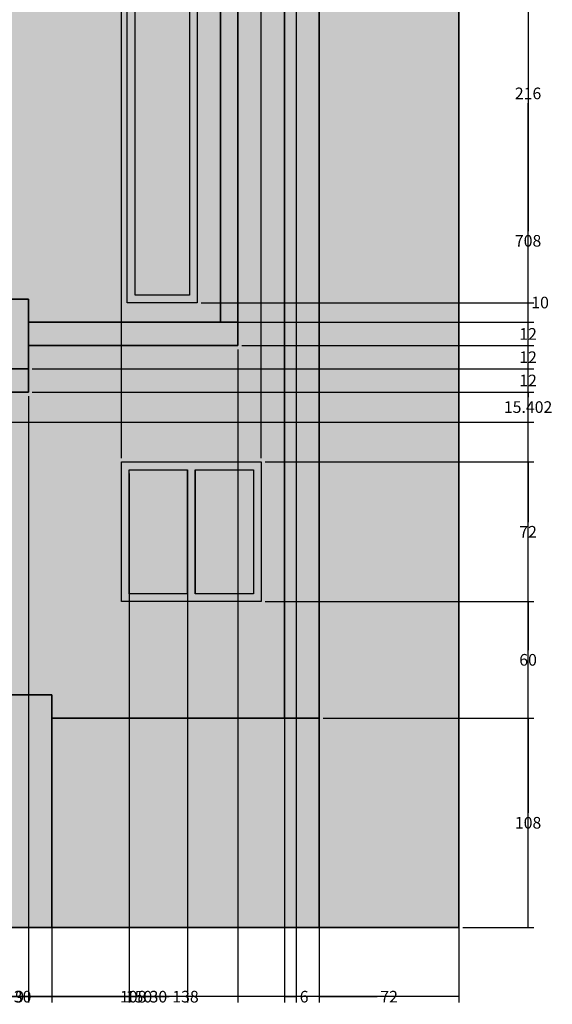
# Model space of a CAD drawing. Units: inches. Extents: x 860 to 1491, y 583 to 1370.
# Tile 6 of 8: x 1216 to 1491, y 583 to 1091. Entities that reach past the tile are written whole.
import ezdxf

# ---------------------------------------------------------------- set-up
doc = ezdxf.new("R2010")
doc.units = ezdxf.units.IN
doc.header["$MEASUREMENT"] = 0
doc.layers.get('0').update_dxf_attribs({"color": 250})
for name, color, linetype, lineweight in [('A-ANNO-DIMS', 2, 'Continuous', 18), ('A-ELEV', 7, 'Continuous', 35), ('A-ELEV-PATT', 9, 'Continuous', 13), ('A-GLAZ', 4, 'Continuous', 25), ('A-GLAZ-PATT', 150, 'Continuous', 13), ('A-SITE-PATT', 8, 'Continuous', 13), ('A-SITE-WALL', 7, 'Continuous', 35)]:
    doc.layers.add(name, color=color, linetype=linetype, lineweight=lineweight)
doc.styles.get("Standard").update_dxf_attribs({"font": 'arial.ttf'})
doc.dimstyles.get("Standard").update_dxf_attribs({"dimtxt": 6, "dimasz": 0.18, "dimexe": 3, "dimexo": 2, "dimgap": 2, "dimtad": 0, "dimtih": 1, "dimtoh": 1, "dimdec": 0, "dimzin": 0, "dimdsep": 46, "dimlunit": 3, "dimtxsty": 'Standard', "dimblk2": 'CLOSEDBLANK', "dimsah": 1, "dimcen": 2, "dimadec": 0, "dimazin": 0, "dimtfac": 1, "dimtdec": 0, "dimtofl": 0, "dimtmove": 0, "dimatfit": 3, "dimfxl": 1, "dimtolj": 1, "dimtzin": 0, "dimarcsym": 0})

# ---------------------------------------------------------------- blocks, each defined once
blk = doc.blocks.new('_ClosedBlank')
at = {"color": 0, "linetype": 'ByBlock', "lineweight": -2}
for p, q in [((-1, 0.17), (0, 0)), ((-1, 0.17), (-1, -0.17)), ((0, 0), (-1, -0.17))]:
    blk.add_line(p, q, dxfattribs=at)
blk = doc.blocks.new('*D2')
at = {"layer": 'A-ANNO-DIMS', "color": 0, "lineweight": -2, "transparency": 16777216}
for p, q in [((1442.44, 1328.76), (1442.44, 584.11)), ((908.34, 740.76), (908.34, 584.11)), ((908.52, 587.11), (1163.85, 587.11)), ((1442.26, 587.11), (1186.93, 587.11))]:
    blk.add_line(p, q, dxfattribs=at)
at = {"layer": 'A-ANNO-DIMS', "color": 0, "transparency": 16777216}
blk.add_solid([(908.52, 587.14), (908.52, 587.08), (908.34, 587.11)], dxfattribs=at)
at = {"layer": 'Defpoints', "color": 0, "transparency": 16777216}
for p in [(1442.44, 1330.76), (908.34, 742.76), (1442.44, 587.11)]:
    blk.add_point(p, dxfattribs=at)
at = {"layer": 'A-ANNO-DIMS', "color": 0, "lineweight": -2, "transparency": 16777216, "xscale": 0.18, "yscale": 0.18, "zscale": 0.18}
blk.add_blockref('_ClosedBlank', (1442.44, 587.11), dxfattribs=at)
at = {"layer": 'A-ANNO-DIMS', "color": 0, "transparency": 16777216, "insert": (1175.39, 587.11), "char_height": 6, "attachment_point": 5}
blk.add_mtext('\\A1;534.1', dxfattribs=at)
blk = doc.blocks.new('*D3')
at = {"layer": 'A-ANNO-DIMS', "color": 0, "lineweight": -2, "transparency": 16777216}
for p, q in [((1444.44, 1330.76), (1481.09, 1330.76)), ((1478.09, 1330.58), (1478.09, 981.82)), ((1478.09, 622.94), (1478.09, 971.69)), ((1444.44, 622.76), (1481.09, 622.76))]:
    blk.add_line(p, q, dxfattribs=at)
at = {"layer": 'A-ANNO-DIMS', "color": 0, "transparency": 16777216}
blk.add_solid([(1478.06, 622.94), (1478.12, 622.94), (1478.09, 622.76)], dxfattribs=at)
at = {"layer": 'Defpoints', "color": 0, "transparency": 16777216}
for p in [(1442.44, 1330.76), (1478.09, 1330.76), (1442.44, 622.76)]:
    blk.add_point(p, dxfattribs=at)
at = {"layer": 'A-ANNO-DIMS', "color": 0, "lineweight": -2, "transparency": 16777216, "xscale": 0.18, "yscale": 0.18, "zscale": 0.18, "rotation": 90}
blk.add_blockref('_ClosedBlank', (1478.09, 1330.76), dxfattribs=at)
at = {"layer": 'A-ANNO-DIMS', "color": 0, "transparency": 16777216, "insert": (1478.09, 976.76), "char_height": 6, "attachment_point": 5}
blk.add_mtext('\\A1;708', dxfattribs=at)
blk = doc.blocks.new('*D17')
at = {"layer": 'A-ANNO-DIMS', "color": 0, "lineweight": -2, "transparency": 16777216}
for p, q in [((1202.44, 740.76), (1202.44, 584.11)), ((1232.44, 740.76), (1232.44, 584.11)), ((1202.62, 587.11), (1211.16, 587.11)), ((1232.26, 587.11), (1223.73, 587.11))]:
    blk.add_line(p, q, dxfattribs=at)
at = {"layer": 'A-ANNO-DIMS', "color": 0, "transparency": 16777216}
blk.add_solid([(1202.62, 587.14), (1202.62, 587.08), (1202.44, 587.11)], dxfattribs=at)
at = {"layer": 'Defpoints', "color": 0, "transparency": 16777216}
for p in [(1202.44, 742.76), (1232.44, 742.76), (1232.44, 587.11)]:
    blk.add_point(p, dxfattribs=at)
at = {"layer": 'A-ANNO-DIMS', "color": 0, "lineweight": -2, "transparency": 16777216, "xscale": 0.18, "yscale": 0.18, "zscale": 0.18}
blk.add_blockref('_ClosedBlank', (1232.44, 587.11), dxfattribs=at)
at = {"layer": 'A-ANNO-DIMS', "color": 0, "transparency": 16777216, "insert": (1217.44, 587.11), "char_height": 6, "attachment_point": 5}
blk.add_mtext('\\A1;30', dxfattribs=at)
blk = doc.blocks.new('*D18')
at = {"layer": 'A-ANNO-DIMS', "color": 0, "lineweight": -2, "transparency": 16777216}
for p, q in [((1232.44, 740.76), (1232.44, 584.11)), ((1370.44, 728.76), (1370.44, 584.11)), ((1232.62, 587.11), (1293.09, 587.11)), ((1370.26, 587.11), (1309.79, 587.11))]:
    blk.add_line(p, q, dxfattribs=at)
at = {"layer": 'A-ANNO-DIMS', "color": 0, "transparency": 16777216}
blk.add_solid([(1232.62, 587.14), (1232.62, 587.08), (1232.44, 587.11)], dxfattribs=at)
at = {"layer": 'Defpoints', "color": 0, "transparency": 16777216}
for p in [(1232.44, 742.76), (1370.44, 730.76), (1370.44, 587.11)]:
    blk.add_point(p, dxfattribs=at)
at = {"layer": 'A-ANNO-DIMS', "color": 0, "lineweight": -2, "transparency": 16777216, "xscale": 0.18, "yscale": 0.18, "zscale": 0.18}
blk.add_blockref('_ClosedBlank', (1370.44, 587.11), dxfattribs=at)
at = {"layer": 'A-ANNO-DIMS', "color": 0, "transparency": 16777216, "insert": (1301.44, 587.11), "char_height": 6, "attachment_point": 5}
blk.add_mtext('\\A1;138', dxfattribs=at)
blk = doc.blocks.new('*D19')
at = {"layer": 'A-ANNO-DIMS', "color": 0, "lineweight": -2, "transparency": 16777216}
for p, q in [((1370.44, 728.76), (1370.44, 584.11)), ((1442.44, 620.76), (1442.44, 584.11)), ((1370.62, 587.11), (1400.2, 587.11)), ((1442.26, 587.11), (1412.68, 587.11))]:
    blk.add_line(p, q, dxfattribs=at)
at = {"layer": 'A-ANNO-DIMS', "color": 0, "transparency": 16777216}
blk.add_solid([(1370.62, 587.14), (1370.62, 587.08), (1370.44, 587.11)], dxfattribs=at)
at = {"layer": 'Defpoints', "color": 0, "transparency": 16777216}
for p in [(1370.44, 730.76), (1442.44, 622.76), (1442.44, 587.11)]:
    blk.add_point(p, dxfattribs=at)
at = {"layer": 'A-ANNO-DIMS', "color": 0, "lineweight": -2, "transparency": 16777216, "xscale": 0.18, "yscale": 0.18, "zscale": 0.18}
blk.add_blockref('_ClosedBlank', (1442.44, 587.11), dxfattribs=at)
at = {"layer": 'A-ANNO-DIMS', "color": 0, "transparency": 16777216, "insert": (1406.44, 587.11), "char_height": 6, "attachment_point": 5}
blk.add_mtext('\\A1;72', dxfattribs=at)
blk = doc.blocks.new('*D26')
at = {"layer": 'A-ANNO-DIMS', "color": 0, "lineweight": -2, "transparency": 16777216}
for p, q in [((1202.44, 744.76), (1202.44, 1369.41)), ((1202.62, 1366.41), (1229.13, 1366.41)), ((1268.26, 1366.41), (1241.75, 1366.41)), ((1268.44, 864.76), (1268.44, 1369.41))]:
    blk.add_line(p, q, dxfattribs=at)
at = {"layer": 'A-ANNO-DIMS', "color": 0, "transparency": 16777216}
blk.add_solid([(1202.62, 1366.44), (1202.62, 1366.38), (1202.44, 1366.41)], dxfattribs=at)
at = {"layer": 'Defpoints', "color": 0, "transparency": 16777216}
for p in [(1268.44, 1366.41), (1268.44, 862.76), (1202.44, 742.76)]:
    blk.add_point(p, dxfattribs=at)
at = {"layer": 'A-ANNO-DIMS', "color": 0, "lineweight": -2, "transparency": 16777216, "xscale": 0.18, "yscale": 0.18, "zscale": 0.18}
blk.add_blockref('_ClosedBlank', (1268.44, 1366.41), dxfattribs=at)
at = {"layer": 'A-ANNO-DIMS', "color": 0, "transparency": 16777216, "insert": (1235.44, 1366.41), "char_height": 6, "attachment_point": 5}
blk.add_mtext('\\A1;66', dxfattribs=at)
blk = doc.blocks.new('*D27')
at = {"layer": 'A-ANNO-DIMS', "color": 0, "lineweight": -2, "transparency": 16777216}
for p, q in [((1268.44, 864.76), (1268.44, 1369.41)), ((1268.62, 1366.41), (1298.2, 1366.41)), ((1340.26, 1366.41), (1310.68, 1366.41)), ((1340.44, 864.76), (1340.44, 1369.41))]:
    blk.add_line(p, q, dxfattribs=at)
at = {"layer": 'A-ANNO-DIMS', "color": 0, "transparency": 16777216}
blk.add_solid([(1268.62, 1366.44), (1268.62, 1366.38), (1268.44, 1366.41)], dxfattribs=at)
at = {"layer": 'Defpoints', "color": 0, "transparency": 16777216}
for p in [(1340.44, 1366.41), (1268.44, 862.76), (1340.44, 862.76)]:
    blk.add_point(p, dxfattribs=at)
at = {"layer": 'A-ANNO-DIMS', "color": 0, "lineweight": -2, "transparency": 16777216, "xscale": 0.18, "yscale": 0.18, "zscale": 0.18}
blk.add_blockref('_ClosedBlank', (1340.44, 1366.41), dxfattribs=at)
at = {"layer": 'A-ANNO-DIMS', "color": 0, "transparency": 16777216, "insert": (1304.44, 1366.41), "char_height": 6, "attachment_point": 5}
blk.add_mtext('\\A1;72', dxfattribs=at)
blk = doc.blocks.new('*D28')
at = {"layer": 'A-ANNO-DIMS', "color": 0, "lineweight": -2, "transparency": 16777216}
for p, q in [((1340.260309, 1366.405507), (1340.080309, 1366.405507)), ((1340.440309, 864.755507), (1340.440309, 1369.405507)), ((1352.440309, 732.755507), (1352.440309, 1369.405507)), ((1352.620309, 1366.405507), (1352.800309, 1366.405507))]:
    blk.add_line(p, q, dxfattribs=at)
at = {"layer": 'A-ANNO-DIMS', "color": 0, "transparency": 16777216}
blk.add_solid([(1340.260309, 1366.435507), (1340.260309, 1366.375507), (1340.440309, 1366.405507)], dxfattribs=at)
at = {"layer": 'Defpoints', "color": 0, "transparency": 16777216}
for p in [(1352.440309, 1366.405507), (1340.440309, 862.755507), (1352.440309, 730.755507)]:
    blk.add_point(p, dxfattribs=at)
at = {"layer": 'A-ANNO-DIMS', "color": 0, "lineweight": -2, "transparency": 16777216, "xscale": 0.18, "yscale": 0.18, "zscale": 0.18, "rotation": 180}
blk.add_blockref('_ClosedBlank', (1352.440309, 1366.405507), dxfattribs=at)
at = {"layer": 'A-ANNO-DIMS', "color": 0, "transparency": 16777216, "insert": (1346.440309, 1366.405507), "char_height": 6, "attachment_point": 5}
blk.add_mtext('\\A1;12', dxfattribs=at)
blk = doc.blocks.new('*D29')
at = {"layer": 'A-ANNO-DIMS', "color": 0, "lineweight": -2, "transparency": 16777216}
for p, q in [((1352.44, 732.76), (1352.44, 1369.41)), ((1352.62, 1366.41), (1355.42, 1366.41)), ((1370.26, 1366.41), (1367.46, 1366.41)), ((1370.44, 732.76), (1370.44, 1369.41))]:
    blk.add_line(p, q, dxfattribs=at)
at = {"layer": 'A-ANNO-DIMS', "color": 0, "transparency": 16777216}
blk.add_solid([(1352.62, 1366.44), (1352.62, 1366.38), (1352.44, 1366.41)], dxfattribs=at)
at = {"layer": 'Defpoints', "color": 0, "transparency": 16777216}
for p in [(1370.44, 1366.41), (1352.44, 730.76), (1370.44, 730.76)]:
    blk.add_point(p, dxfattribs=at)
at = {"layer": 'A-ANNO-DIMS', "color": 0, "lineweight": -2, "transparency": 16777216, "xscale": 0.18, "yscale": 0.18, "zscale": 0.18}
blk.add_blockref('_ClosedBlank', (1370.44, 1366.41), dxfattribs=at)
at = {"layer": 'A-ANNO-DIMS', "color": 0, "transparency": 16777216, "insert": (1361.44, 1366.41), "char_height": 6, "attachment_point": 5}
blk.add_mtext('\\A1;18', dxfattribs=at)
blk = doc.blocks.new('*D30')
at = {"layer": 'A-ANNO-DIMS', "color": 0, "lineweight": -2, "transparency": 16777216}
for p, q in [((1272.44, 856.76), (1272.44, 584.11)), ((1302.44, 856.76), (1302.44, 584.11)), ((1272.62, 587.11), (1281.16, 587.11)), ((1302.26, 587.11), (1293.73, 587.11))]:
    blk.add_line(p, q, dxfattribs=at)
at = {"layer": 'A-ANNO-DIMS', "color": 0, "transparency": 16777216}
blk.add_solid([(1272.62, 587.14), (1272.62, 587.08), (1272.44, 587.11)], dxfattribs=at)
at = {"layer": 'Defpoints', "color": 0, "transparency": 16777216}
for p in [(1272.44, 858.76), (1302.44, 858.76), (1302.44, 587.11)]:
    blk.add_point(p, dxfattribs=at)
at = {"layer": 'A-ANNO-DIMS', "color": 0, "lineweight": -2, "transparency": 16777216, "xscale": 0.18, "yscale": 0.18, "zscale": 0.18}
blk.add_blockref('_ClosedBlank', (1302.44, 587.11), dxfattribs=at)
at = {"layer": 'A-ANNO-DIMS', "color": 0, "transparency": 16777216, "insert": (1287.44, 587.11), "char_height": 6, "attachment_point": 5}
blk.add_mtext('\\A1;30', dxfattribs=at)
blk = doc.blocks.new('*D36')
at = {"layer": 'A-ANNO-DIMS', "color": 0, "lineweight": -2, "transparency": 16777216}
for p, q in [((1372.44, 730.76), (1481.09, 730.76)), ((1478.09, 730.58), (1478.09, 681.82)), ((1478.09, 622.94), (1478.09, 671.69)), ((1444.44, 622.76), (1481.09, 622.76))]:
    blk.add_line(p, q, dxfattribs=at)
at = {"layer": 'A-ANNO-DIMS', "color": 0, "transparency": 16777216}
blk.add_solid([(1478.06, 622.94), (1478.12, 622.94), (1478.09, 622.76)], dxfattribs=at)
at = {"layer": 'Defpoints', "color": 0, "transparency": 16777216}
for p in [(1370.44, 730.76), (1478.09, 730.76), (1442.44, 622.76)]:
    blk.add_point(p, dxfattribs=at)
at = {"layer": 'A-ANNO-DIMS', "color": 0, "lineweight": -2, "transparency": 16777216, "xscale": 0.18, "yscale": 0.18, "zscale": 0.18, "rotation": 90}
blk.add_blockref('_ClosedBlank', (1478.09, 730.76), dxfattribs=at)
at = {"layer": 'A-ANNO-DIMS', "color": 0, "transparency": 16777216, "insert": (1478.09, 676.76), "char_height": 6, "attachment_point": 5}
blk.add_mtext('\\A1;108', dxfattribs=at)
blk = doc.blocks.new('*D37')
at = {"layer": 'A-ANNO-DIMS', "color": 0, "lineweight": -2, "transparency": 16777216}
for p, q in [((1342.44, 790.76), (1481.09, 790.76)), ((1478.09, 790.58), (1478.09, 765.82)), ((1478.09, 730.94), (1478.09, 755.69)), ((1372.44, 730.76), (1481.09, 730.76))]:
    blk.add_line(p, q, dxfattribs=at)
at = {"layer": 'A-ANNO-DIMS', "color": 0, "transparency": 16777216}
blk.add_solid([(1478.06, 730.94), (1478.12, 730.94), (1478.09, 730.76)], dxfattribs=at)
at = {"layer": 'Defpoints', "color": 0, "transparency": 16777216}
for p in [(1340.44, 790.76), (1478.09, 790.76), (1370.44, 730.76)]:
    blk.add_point(p, dxfattribs=at)
at = {"layer": 'A-ANNO-DIMS', "color": 0, "lineweight": -2, "transparency": 16777216, "xscale": 0.18, "yscale": 0.18, "zscale": 0.18, "rotation": 90}
blk.add_blockref('_ClosedBlank', (1478.09, 790.76), dxfattribs=at)
at = {"layer": 'A-ANNO-DIMS', "color": 0, "transparency": 16777216, "insert": (1478.09, 760.76), "char_height": 6, "attachment_point": 5}
blk.add_mtext('\\A1;60', dxfattribs=at)
blk = doc.blocks.new('*D38')
at = {"layer": 'A-ANNO-DIMS', "color": 0, "lineweight": -2, "transparency": 16777216}
for p, q in [((1342.44, 862.76), (1481.09, 862.76)), ((1478.09, 862.58), (1478.09, 831.77)), ((1478.09, 790.94), (1478.09, 821.74)), ((1342.44, 790.76), (1481.09, 790.76))]:
    blk.add_line(p, q, dxfattribs=at)
at = {"layer": 'A-ANNO-DIMS', "color": 0, "transparency": 16777216}
blk.add_solid([(1478.06, 790.94), (1478.12, 790.94), (1478.09, 790.76)], dxfattribs=at)
at = {"layer": 'Defpoints', "color": 0, "transparency": 16777216}
for p in [(1340.44, 862.76), (1478.09, 862.76), (1340.44, 790.76)]:
    blk.add_point(p, dxfattribs=at)
at = {"layer": 'A-ANNO-DIMS', "color": 0, "lineweight": -2, "transparency": 16777216, "xscale": 0.18, "yscale": 0.18, "zscale": 0.18, "rotation": 90}
blk.add_blockref('_ClosedBlank', (1478.09, 862.76), dxfattribs=at)
at = {"layer": 'A-ANNO-DIMS', "color": 0, "transparency": 16777216, "insert": (1478.09, 826.76), "char_height": 6, "attachment_point": 5}
blk.add_mtext('\\A1;72', dxfattribs=at)
blk = doc.blocks.new('*D48')
at = {"layer": 'A-ANNO-DIMS', "color": 0, "lineweight": -2, "transparency": 16777216}
for p, q in [((1222.44, 898.76), (1481.09, 898.76)), ((1478.09, 898.58), (1478.09, 896.12)), ((964.34, 883.35), (1481.09, 883.35)), ((1478.09, 883.53), (1478.09, 885.99))]:
    blk.add_line(p, q, dxfattribs=at)
at = {"layer": 'A-ANNO-DIMS', "color": 0, "transparency": 16777216}
blk.add_solid([(1478.06, 883.53), (1478.12, 883.53), (1478.09, 883.35)], dxfattribs=at)
at = {"layer": 'Defpoints', "color": 0, "transparency": 16777216}
for p in [(1220.44, 898.76), (1478.09, 898.76), (962.34, 883.35)]:
    blk.add_point(p, dxfattribs=at)
at = {"layer": 'A-ANNO-DIMS', "color": 0, "lineweight": -2, "transparency": 16777216, "xscale": 0.18, "yscale": 0.18, "zscale": 0.18, "rotation": 90}
blk.add_blockref('_ClosedBlank', (1478.09, 898.76), dxfattribs=at)
at = {"layer": 'A-ANNO-DIMS', "color": 0, "transparency": 16777216, "insert": (1478.09, 891.05), "char_height": 6, "attachment_point": 5}
blk.add_mtext('\\A1;15.402', dxfattribs=at)
blk = doc.blocks.new('*D49')
at = {"layer": 'A-ANNO-DIMS', "color": 0, "lineweight": -2, "transparency": 16777216}
for p, q in [((1222.440309, 910.755507), (1481.090309, 910.755507)), ((1478.090309, 910.935507), (1478.090309, 911.115507)), ((1222.440309, 898.755507), (1481.090309, 898.755507)), ((1478.090309, 898.575507), (1478.090309, 898.395507))]:
    blk.add_line(p, q, dxfattribs=at)
at = {"layer": 'A-ANNO-DIMS', "color": 0, "transparency": 16777216}
blk.add_solid([(1478.060309, 898.575507), (1478.120309, 898.575507), (1478.090309, 898.755507)], dxfattribs=at)
at = {"layer": 'Defpoints', "color": 0, "transparency": 16777216}
for p in [(1220.440309, 910.755507), (1478.090309, 910.755507), (1220.440309, 898.755507)]:
    blk.add_point(p, dxfattribs=at)
at = {"layer": 'A-ANNO-DIMS', "color": 0, "lineweight": -2, "transparency": 16777216, "xscale": 0.18, "yscale": 0.18, "zscale": 0.18, "rotation": 270}
blk.add_blockref('_ClosedBlank', (1478.090309, 910.755507), dxfattribs=at)
at = {"layer": 'A-ANNO-DIMS', "color": 0, "transparency": 16777216, "insert": (1478.090309, 904.755507), "char_height": 6, "attachment_point": 5}
blk.add_mtext('\\A1;12', dxfattribs=at)
blk = doc.blocks.new('*D50')
at = {"layer": 'A-ANNO-DIMS', "color": 0, "lineweight": -2, "transparency": 16777216}
for p, q in [((1330.440309, 922.755507), (1481.090309, 922.755507)), ((1478.090309, 922.935507), (1478.090309, 923.115507)), ((1222.440309, 910.755507), (1481.090309, 910.755507)), ((1478.090309, 910.575507), (1478.090309, 910.395507))]:
    blk.add_line(p, q, dxfattribs=at)
at = {"layer": 'A-ANNO-DIMS', "color": 0, "transparency": 16777216}
blk.add_solid([(1478.060309, 910.575507), (1478.120309, 910.575507), (1478.090309, 910.755507)], dxfattribs=at)
at = {"layer": 'Defpoints', "color": 0, "transparency": 16777216}
for p in [(1328.440309, 922.755507), (1478.090309, 922.755507), (1220.440309, 910.755507)]:
    blk.add_point(p, dxfattribs=at)
at = {"layer": 'A-ANNO-DIMS', "color": 0, "lineweight": -2, "transparency": 16777216, "xscale": 0.18, "yscale": 0.18, "zscale": 0.18, "rotation": 270}
blk.add_blockref('_ClosedBlank', (1478.090309, 922.755507), dxfattribs=at)
at = {"layer": 'A-ANNO-DIMS', "color": 0, "transparency": 16777216, "insert": (1478.090309, 916.755507), "char_height": 6, "attachment_point": 5}
blk.add_mtext('\\A1;12', dxfattribs=at)
blk = doc.blocks.new('*D51')
at = {"layer": 'A-ANNO-DIMS', "color": 0, "lineweight": -2, "transparency": 16777216}
for p, q in [((1321.440309, 934.755507), (1481.090309, 934.755507)), ((1478.090309, 934.935507), (1478.090309, 935.115507)), ((1330.440309, 922.755507), (1481.090309, 922.755507)), ((1478.090309, 922.575507), (1478.090309, 922.395507))]:
    blk.add_line(p, q, dxfattribs=at)
at = {"layer": 'A-ANNO-DIMS', "color": 0, "transparency": 16777216}
blk.add_solid([(1478.060309, 922.575507), (1478.120309, 922.575507), (1478.090309, 922.755507)], dxfattribs=at)
at = {"layer": 'Defpoints', "color": 0, "transparency": 16777216}
for p in [(1319.440309, 934.755507), (1478.090309, 934.755507), (1328.440309, 922.755507)]:
    blk.add_point(p, dxfattribs=at)
at = {"layer": 'A-ANNO-DIMS', "color": 0, "lineweight": -2, "transparency": 16777216, "xscale": 0.18, "yscale": 0.18, "zscale": 0.18, "rotation": 270}
blk.add_blockref('_ClosedBlank', (1478.090309, 934.755507), dxfattribs=at)
at = {"layer": 'A-ANNO-DIMS', "color": 0, "transparency": 16777216, "insert": (1478.090309, 928.755507), "char_height": 6, "attachment_point": 5}
blk.add_mtext('\\A1;12', dxfattribs=at)
blk = doc.blocks.new('*D52')
at = {"layer": 'A-ANNO-DIMS', "color": 0, "lineweight": -2, "transparency": 16777216}
for p, q in [((1309.44, 944.76), (1481.09, 944.76)), ((1478.09, 944.76), (1478.09, 944.94)), ((1478.09, 944.94), (1478.27, 944.94)), ((1478.09, 934.94), (1478.09, 944.58)), ((1321.44, 934.76), (1481.09, 934.76))]:
    blk.add_line(p, q, dxfattribs=at)
at = {"layer": 'A-ANNO-DIMS', "color": 0, "transparency": 16777216}
blk.add_solid([(1478.06, 934.94), (1478.12, 934.94), (1478.09, 934.76)], dxfattribs=at)
at = {"layer": 'Defpoints', "color": 0, "transparency": 16777216}
for p in [(1307.44, 944.76), (1478.09, 944.76), (1319.44, 934.76)]:
    blk.add_point(p, dxfattribs=at)
at = {"layer": 'A-ANNO-DIMS', "color": 0, "lineweight": -2, "transparency": 16777216, "xscale": 0.18, "yscale": 0.18, "zscale": 0.18, "rotation": 90}
blk.add_blockref('_ClosedBlank', (1478.09, 944.76), dxfattribs=at)
at = {"layer": 'A-ANNO-DIMS', "color": 0, "transparency": 16777216, "insert": (1484.28, 944.94), "char_height": 6, "attachment_point": 5}
blk.add_mtext('\\A1;10', dxfattribs=at)
blk = doc.blocks.new('*D53')
at = {"layer": 'A-ANNO-DIMS', "color": 0, "lineweight": -2, "transparency": 16777216}
for p, q in [((1309.44, 1160.76), (1481.09, 1160.76)), ((1478.09, 1160.58), (1478.09, 1057.82)), ((1478.09, 944.94), (1478.09, 1047.69)), ((1309.44, 944.76), (1481.09, 944.76))]:
    blk.add_line(p, q, dxfattribs=at)
at = {"layer": 'A-ANNO-DIMS', "color": 0, "transparency": 16777216}
blk.add_solid([(1478.06, 944.94), (1478.12, 944.94), (1478.09, 944.76)], dxfattribs=at)
at = {"layer": 'Defpoints', "color": 0, "transparency": 16777216}
for p in [(1307.44, 1160.76), (1478.09, 1160.76), (1307.44, 944.76)]:
    blk.add_point(p, dxfattribs=at)
at = {"layer": 'A-ANNO-DIMS', "color": 0, "lineweight": -2, "transparency": 16777216, "xscale": 0.18, "yscale": 0.18, "zscale": 0.18, "rotation": 90}
blk.add_blockref('_ClosedBlank', (1478.09, 1160.76), dxfattribs=at)
at = {"layer": 'A-ANNO-DIMS', "color": 0, "transparency": 16777216, "insert": (1478.09, 1052.76), "char_height": 6, "attachment_point": 5}
blk.add_mtext('\\A1;216', dxfattribs=at)
blk = doc.blocks.new('*D61')
at = {"layer": 'A-ANNO-DIMS', "color": 0, "lineweight": -2, "transparency": 16777216}
for p, q in [((1319.260309, 1366.405507), (1319.080309, 1366.405507)), ((1319.440309, 1186.755507), (1319.440309, 1369.405507)), ((1328.440309, 924.755507), (1328.440309, 1369.405507)), ((1328.620309, 1366.405507), (1328.800309, 1366.405507))]:
    blk.add_line(p, q, dxfattribs=at)
at = {"layer": 'A-ANNO-DIMS', "color": 0, "transparency": 16777216}
blk.add_solid([(1319.260309, 1366.435507), (1319.260309, 1366.375507), (1319.440309, 1366.405507)], dxfattribs=at)
at = {"layer": 'Defpoints', "color": 0, "transparency": 16777216}
for p in [(1328.440309, 1366.405507), (1319.440309, 1184.755507), (1328.440309, 922.755507)]:
    blk.add_point(p, dxfattribs=at)
at = {"layer": 'A-ANNO-DIMS', "color": 0, "lineweight": -2, "transparency": 16777216, "xscale": 0.18, "yscale": 0.18, "zscale": 0.18, "rotation": 180}
blk.add_blockref('_ClosedBlank', (1328.440309, 1366.405507), dxfattribs=at)
at = {"layer": 'A-ANNO-DIMS', "color": 0, "transparency": 16777216, "insert": (1323.940309, 1366.405507), "char_height": 6, "attachment_point": 5}
blk.add_mtext('\\A1;9', dxfattribs=at)
blk = doc.blocks.new('*D69')
at = {"layer": 'A-ANNO-DIMS', "color": 0, "lineweight": -2, "transparency": 16777216}
for p, q in [((1211.440309, 980.755507), (1211.440309, 584.105507)), ((1220.440309, 896.755507), (1220.440309, 584.105507)), ((1211.260309, 587.105507), (1211.080309, 587.105507)), ((1220.620309, 587.105507), (1220.800309, 587.105507))]:
    blk.add_line(p, q, dxfattribs=at)
at = {"layer": 'A-ANNO-DIMS', "color": 0, "transparency": 16777216}
blk.add_solid([(1211.260309, 587.135507), (1211.260309, 587.075507), (1211.440309, 587.105507)], dxfattribs=at)
at = {"layer": 'Defpoints', "color": 0, "transparency": 16777216}
for p in [(1211.440309, 982.755507), (1220.440309, 898.755507), (1220.440309, 587.105507)]:
    blk.add_point(p, dxfattribs=at)
at = {"layer": 'A-ANNO-DIMS', "color": 0, "lineweight": -2, "transparency": 16777216, "xscale": 0.18, "yscale": 0.18, "zscale": 0.18, "rotation": 180}
blk.add_blockref('_ClosedBlank', (1220.440309, 587.105507), dxfattribs=at)
at = {"layer": 'A-ANNO-DIMS', "color": 0, "transparency": 16777216, "insert": (1215.940309, 587.105507), "char_height": 6, "attachment_point": 5}
blk.add_mtext('\\A1;9', dxfattribs=at)
blk = doc.blocks.new('*D70')
at = {"layer": 'A-ANNO-DIMS', "color": 0, "lineweight": -2, "transparency": 16777216}
for p, q in [((1328.44, 920.76), (1328.44, 584.11)), ((1220.44, 896.76), (1220.44, 584.11)), ((1220.62, 587.11), (1266.09, 587.11)), ((1328.26, 587.11), (1282.79, 587.11))]:
    blk.add_line(p, q, dxfattribs=at)
at = {"layer": 'A-ANNO-DIMS', "color": 0, "transparency": 16777216}
blk.add_solid([(1220.62, 587.14), (1220.62, 587.08), (1220.44, 587.11)], dxfattribs=at)
at = {"layer": 'Defpoints', "color": 0, "transparency": 16777216}
for p in [(1328.44, 922.76), (1220.44, 898.76), (1328.44, 587.11)]:
    blk.add_point(p, dxfattribs=at)
at = {"layer": 'A-ANNO-DIMS', "color": 0, "lineweight": -2, "transparency": 16777216, "xscale": 0.18, "yscale": 0.18, "zscale": 0.18}
blk.add_blockref('_ClosedBlank', (1328.44, 587.11), dxfattribs=at)
at = {"layer": 'A-ANNO-DIMS', "color": 0, "transparency": 16777216, "insert": (1274.44, 587.11), "char_height": 6, "attachment_point": 5}
blk.add_mtext('\\A1;108', dxfattribs=at)
blk = doc.blocks.new('*D77')
at = {"layer": 'A-ANNO-DIMS', "color": 0, "lineweight": -2, "transparency": 16777216}
for p, q in [((1202.44, 1277.76), (1202.44, 584.11)), ((1352.44, 1277.76), (1352.44, 584.11)), ((1202.62, 587.11), (1269.1, 587.11)), ((1352.26, 587.11), (1285.78, 587.11))]:
    blk.add_line(p, q, dxfattribs=at)
at = {"layer": 'A-ANNO-DIMS', "color": 0, "transparency": 16777216}
blk.add_solid([(1202.62, 587.14), (1202.62, 587.08), (1202.44, 587.11)], dxfattribs=at)
at = {"layer": 'Defpoints', "color": 0, "transparency": 16777216}
for p in [(1202.44, 1279.76), (1352.44, 1279.76), (1352.44, 587.11)]:
    blk.add_point(p, dxfattribs=at)
at = {"layer": 'A-ANNO-DIMS', "color": 0, "lineweight": -2, "transparency": 16777216, "xscale": 0.18, "yscale": 0.18, "zscale": 0.18}
blk.add_blockref('_ClosedBlank', (1352.44, 587.11), dxfattribs=at)
at = {"layer": 'A-ANNO-DIMS', "color": 0, "transparency": 16777216, "insert": (1277.44, 587.11), "char_height": 6, "attachment_point": 5}
blk.add_mtext('\\A1;150', dxfattribs=at)
blk = doc.blocks.new('*D78')
at = {"layer": 'A-ANNO-DIMS', "color": 0, "lineweight": -2, "transparency": 16777216}
for p, q in [((1358.44, 1286.76), (1358.44, 584.11)), ((1352.44, 1277.76), (1352.44, 584.11)), ((1352.62, 587.11), (1358.26, 587.11)), ((1358.44, 587.11), (1358.62, 587.11))]:
    blk.add_line(p, q, dxfattribs=at)
at = {"layer": 'A-ANNO-DIMS', "color": 0, "transparency": 16777216}
blk.add_solid([(1352.62, 587.14), (1352.62, 587.08), (1352.44, 587.11)], dxfattribs=at)
at = {"layer": 'Defpoints', "color": 0, "transparency": 16777216}
for p in [(1358.44, 1288.76), (1352.44, 1279.76), (1358.44, 587.11)]:
    blk.add_point(p, dxfattribs=at)
at = {"layer": 'A-ANNO-DIMS', "color": 0, "lineweight": -2, "transparency": 16777216, "xscale": 0.18, "yscale": 0.18, "zscale": 0.18}
blk.add_blockref('_ClosedBlank', (1358.44, 587.11), dxfattribs=at)
at = {"layer": 'A-ANNO-DIMS', "color": 0, "transparency": 16777216, "insert": (1362.6, 587.11), "char_height": 6, "attachment_point": 5}
blk.add_mtext('\\A1;6', dxfattribs=at)

msp = doc.modelspace()

# ---------------------------------------------------------------- hatches: boundary and pattern name
at = {"layer": 'A-ELEV-PATT'}
h = msp.add_hatch(color=256, dxfattribs=at)
h.dxf.hatch_style = 1
h.paths.add_polyline_path([(1442.4403, 1330.7555), (1370.4403, 1330.7555), (1370.4403, 622.7555), (1442.4403, 622.7555)])
h.paths.add_polyline_path([(1358.4403, 1306.7555), (1190.4403, 1306.7555), (1190.4403, 1288.7555), (1358.4403, 1288.7555)])
h.paths.add_polyline_path([(1190.4403, 1234.7555), (962.3403, 1234.7555), (962.3403, 1198.7555), (1202.4403, 1198.7555), (1202.4403, 1216.7555), (1190.4403, 1216.7555)])
h.paths.add_polyline_path([(1202.4403, 1117.6207), (962.3403, 1117.6207), (962.3403, 982.7555), (986.3403, 982.7555), (986.3403, 1090.7555), (1178.3403, 1090.7555), (1178.3403, 982.7555), (1202.4403, 982.7555)])
h.paths.add_polyline_path([(1319.4403, 1184.7555), (1202.4403, 1184.7555), (1202.4403, 982.7555), (1211.4403, 982.7555), (1211.4403, 946.7555), (1220.4403, 946.7555), (1220.4403, 934.7555), (1319.4403, 934.7555)])
h.paths.add_polyline_path([(1271.4403, 1160.7555), (1307.4403, 1160.7555), (1307.4403, 944.7555), (1271.4403, 944.7555)], flags=16)
h.paths.add_polyline_path([(1275.4403, 1156.7555), (1303.4403, 1156.7555), (1303.4403, 948.7555), (1275.4403, 948.7555)], flags=0)
h.paths.add_polyline_path([(1202.4403, 898.7555), (962.3403, 898.7555), (962.3403, 730.7555), (1034.4585, 730.7555), (1034.4585, 826.7555), (1070.4585, 826.7555), (1070.4585, 730.7555), (1118.4403, 730.7555), (1118.4403, 838.7555), (1178.4403, 838.7555), (1178.4403, 730.7555), (1202.4403, 730.7555)])
h.paths.add_polyline_path([(1220.4403, 946.7555), (1211.4403, 946.7555), (938.3403, 946.7555), (926.3403, 946.7555), (926.3403, 910.7555), (962.3403, 910.7555), (1220.4403, 910.7555)])
h.paths.add_polyline_path([(950.3403, 730.7555), (950.3403, 734.7555), (938.3403, 742.7555), (938.3403, 730.7555), (938.3403, 622.7555), (950.3403, 622.7555)])
h = msp.add_hatch(color=256, dxfattribs=at)
h.dxf.hatch_style = 1
h.paths.add_polyline_path([(1202.4403, 1184.7555), (1319.4403, 1184.7555), (1328.4403, 1189.7555), (938.3403, 1189.7555), (962.3403, 1098.3061), (962.3403, 1117.6207), (1202.4403, 1117.6207)])
h.paths.add_polyline_path([(1202.4403, 1198.7555), (938.3403, 1198.7555), (938.3403, 1189.7555), (1202.4403, 1189.7555)])
h.paths.add_polyline_path([(1328.4403, 1198.7555), (1202.4403, 1198.7555), (1202.4403, 1189.7555), (1328.4403, 1189.7555)])
h.paths.add_polyline_path([(1328.4403, 1189.7555), (1319.4403, 1184.7555), (1319.4403, 934.7555), (1328.4403, 934.7555)])
h.paths.add_polyline_path([(1328.4403, 934.7555), (1319.4403, 934.7555), (1220.4403, 934.7555), (1220.4403, 922.7555), (1328.4403, 922.7555)])
h.paths.add_polyline_path([(1202.4403, 1279.7555), (1190.4403, 1279.7555), (1190.4403, 1216.7555), (1202.4403, 1216.7555)])
h.paths.add_polyline_path([(1358.4403, 1288.7555), (1190.4403, 1288.7555), (1190.4403, 1279.7555), (1352.4403, 1279.7555)])
h.paths.add_polyline_path([(1370.4403, 1330.7555), (1352.4403, 1318.7555), (1352.4403, 1306.7555), (1358.4403, 1306.7555), (1358.4403, 1288.7555), (1352.4403, 1279.7555), (1352.4403, 730.7555), (1370.4403, 730.7555)])
h = msp.add_hatch(color=256, dxfattribs=at)
h.dxf.hatch_style = 1
h.paths.add_polyline_path([(1352.4403, 1279.7555), (1202.4403, 1279.7555), (1202.4403, 1198.7555), (1328.4403, 1198.7555), (1328.4403, 922.7555), (1220.4403, 922.7555), (1220.4403, 898.7555), (1202.4403, 898.7555), (1202.4403, 742.7555), (1232.4403, 742.7555), (1232.4403, 730.7555), (1352.4403, 730.7555)])
h.paths.add_polyline_path([(1268.4403, 862.7555), (1340.4403, 862.7555), (1340.4403, 790.7555), (1268.4403, 790.7555)], flags=16)
h.paths.add_polyline_path([(1272.4403, 858.7555), (1302.4403, 858.7555), (1302.4403, 794.7555), (1272.4403, 794.7555)], flags=0)
h.paths.add_polyline_path([(1306.4403, 858.7555), (1336.4403, 858.7555), (1336.4403, 794.7555), (1306.4403, 794.7555)], flags=0)
h = msp.add_hatch(color=256, dxfattribs=at)
h.paths.add_polyline_path([(1176.3403, 1088.7555), (988.3403, 1088.7555), (988.3403, 982.7555), (998.3403, 982.7555), (998.3403, 1078.7555), (1079.3403, 1078.7555), (1079.3403, 982.7555), (1085.3403, 982.7555), (1085.3403, 1078.7555), (1166.3403, 1078.7555), (1166.3403, 982.7555), (1176.3403, 982.7555)])
h.paths.add_polyline_path([(1176.3403, 982.7555), (1166.3403, 982.7555), (1166.3403, 958.7555), (1085.3403, 958.7555), (1085.3403, 982.7555), (1079.3403, 982.7555), (1079.3403, 958.7555), (998.3403, 958.7555), (998.3403, 982.7555), (988.3403, 982.7555), (988.3403, 948.7555), (1176.3403, 948.7555)])
h.paths.add_polyline_path([(1307.4403, 1160.7555), (1271.4403, 1160.7555), (1271.4403, 944.7555), (1307.4403, 944.7555)])
h.paths.add_polyline_path([(1275.4403, 1156.7555), (1303.4403, 1156.7555), (1303.4403, 948.7555), (1275.4403, 948.7555)], flags=16)
h.paths.add_polyline_path([(1340.4403, 862.7555), (1268.4403, 862.7555), (1268.4403, 790.7555), (1340.4403, 790.7555)])
h.paths.add_polyline_path([(1306.4403, 794.7555), (1306.4403, 858.7555), (1336.4403, 858.7555), (1336.4403, 794.7555)], flags=16)
h.paths.add_polyline_path([(1302.4403, 794.7555), (1272.4403, 794.7555), (1272.4403, 858.7555), (1302.4403, 858.7555)], flags=16)
h.paths.add_polyline_path([(1124.4403, 832.7555), (1172.4403, 832.7555), (1172.4403, 730.7555), (1178.4403, 730.7555), (1178.4403, 838.7555), (1118.4403, 838.7555), (1118.4403, 742.7555), (1124.4403, 742.7555), (1124.4403, 766.7555)])
h.paths.add_polyline_path([(1070.4585, 826.7555), (1034.4585, 826.7555), (1034.4585, 730.7555), (1070.4585, 730.7555)])
h.paths.add_polyline_path([(1066.4585, 822.7555), (1066.4585, 734.7555), (1038.4585, 734.7555), (1038.4585, 822.7555)], flags=16)
h.paths.add_polyline_path([(1129.9403, 766.7555, 1), (1124.9403, 766.7555, 1)], flags=17)
h = msp.add_hatch(color=256, dxfattribs=at)
h.dxf.hatch_style = 1
h.paths.add_polyline_path([(1220.4403, 910.7555), (938.3403, 910.7555), (926.3403, 910.7555), (962.3403, 883.3536), (962.3403, 898.7555), (1220.4403, 898.7555)])
h = msp.add_hatch(color=256, dxfattribs=at)
h.dxf.hatch_style = 1
h.paths.add_polyline_path([(1370.4403, 730.7555), (1232.4403, 730.7555), (1232.4403, 622.7555), (1370.4403, 622.7555)])
h.paths.add_polyline_path([(1232.4403, 730.7555), (1232.4403, 742.7555), (1202.4403, 742.7555), (1202.4403, 622.7555), (1232.4403, 622.7555)])
h.paths.add_polyline_path([(1148.4403, 730.7555), (1148.4403, 742.7555), (1118.4403, 742.7555), (1118.4403, 718.7555), (1118.4403, 622.7555), (1148.4403, 622.7555)])
h.paths.add_polyline_path([(938.3403, 730.7555), (938.3403, 742.7555), (908.3403, 742.7555), (908.3403, 736.7555), (908.3403, 622.7555), (938.3403, 622.7555)])
at = {"layer": 'A-GLAZ-PATT'}
h = msp.add_hatch(color=256, dxfattribs=at)
h.set_gradient(color1=(51, 167, 230), color2=(122, 175, 223), name='CYLINDER')
h.paths.add_polyline_path([(1275.4403, 948.7555), (1303.4403, 948.7555), (1303.4403, 1156.7555), (1275.4403, 1156.7555)])
h = msp.add_hatch(color=256, dxfattribs=at)
h.set_gradient(color1=(51, 167, 230), color2=(122, 175, 223), name='CYLINDER')
h.paths.add_polyline_path([(1272.4403, 794.7555), (1302.4403, 794.7555), (1302.4403, 858.7555), (1272.4403, 858.7555)])
h = msp.add_hatch(color=256, dxfattribs=at)
h.set_gradient(color1=(51, 167, 230), color2=(122, 175, 223), name='CYLINDER')
h.paths.add_polyline_path([(1306.4403, 794.7555), (1336.4403, 794.7555), (1336.4403, 858.7555), (1306.4403, 858.7555)])
at = {"layer": 'A-SITE-PATT'}
h = msp.add_hatch(dxfattribs=at)
h.set_pattern_fill('GRAVEL', color=256, scale=30, style=0)
h.set_pattern_definition([(228.01279, (21.6, 30), (-240, -270), [4.0361, -399.57264]), (184.96974, (18.9, 27), (360, 30), [6.92604, -685.67774]), (132.51045, (12, 26.4), (300, -330), [4.88364, -483.481]), (267.27369, (0.3, 18.9), (30, 600), [6.30714, -624.40674]), (292.83365, (0, 12.6), (-150, 360), [6.18465, -612.2812]), (357.27369, (2.4, 6.9), (-600, 30), [6.30714, -624.40674]), (37.69424, (8.7, 6.6), (-390, -300), [8.34087, -825.74546]), (72.25533, (15.3, 11.7), (210, 660), [7.87464, -779.58964]), (121.42957, (17.7, 19.2), (-240, 390), [6.3285, -626.5222]), (175.23636, (14.4, 24.6), (330, -30), [7.22496, -354.0229]), (222.39744, (7.2, 25.2), (-360, -330), [9.34344, -925.00125]), (138.81407, (30, 18.6), (-210, 180), [3.18903, -315.71534]), (171.46923, (27.6, 20.7), (390, -60), [6.0671, -600.64534]), (225, (21.6, 21.6), (-3e-15, -30), [4.24263, -38.1838]), (203.1986, (19.5, 25.2), (150, 60), [2.28474, -226.18845]), (291.8014, (17.4, 24.3), (-30, 90), [3.2311, -158.32385]), (30.96376, (18.6, 21.3), (90, 60), [5.24787, -169.6807]), (161.56505, (23.1, 24), (60, -30), [3.79473, -91.0736]), (16.38954, (0, 24.3), (300, 90), [5.316, -526.28535]), (70.34618, (5.1, 25.8), (-120, -330), [4.45983, -441.52223]), (293.1986, (23.1, 30), (-60, 150), [4.56945, -223.90374]), (343.61046, (24.9, 25.8), (-300, 90), [5.316, -526.28535]), (339.44395, (0, 5.7), (-150, 60), [5.1264, -251.1937]), (294.77514, (4.8, 3.9), (-150, 330), [4.29534, -425.2393]), (66.8014, (23.4, 0), (60, 150), [4.56945, -223.90374]), (17.35402, (25.2, 4.2), (-390, -120), [5.02893, -497.8627]), (69.44395, (8.7, 0), (-60, -150), [2.5632, -253.7569]), (101.30993, (21.6, 0), (-30, 120), [1.5297, -151.4409]), (165.96376, (21.3, 1.5), (90, -30), [6.18465, -117.5085]), (186.00901, (15.3, 3), (300, 30), [5.7315, -567.4177]), (303.69007, (18.6, 18.6), (-30, 60), [4.32666, -103.8399]), (353.15723, (21, 15), (510, -60), [7.55382, -747.82688]), (60.9454, (28.5, 14.1), (-120, -210), [3.0887, -305.7802]), (90, (30, 16.8), (-30, 30), [1.8, -28.2]), (120.25644, (14.7, 3.9), (120, -210), [4.1677, -412.6056]), (48.01279, (12.6, 7.5), (240, 270), [8.07216, -395.53656]), (0, (18, 13.5), (30, 30), [7.8, -22.2]), (325.30485, (25.8, 13.5), (300, -210), [4.7434, -469.59823]), (254.0546, (29.7, 10.8), (-30, -120), [4.36806, -214.03524]), (207.64598, (28.5, 6.6), (-570, -300), [7.11195, -704.08423]), (175.42608, (22.2, 3.3), (-390, 30), [7.52397, -744.8722])])
h.paths.add_polyline_path([(1370.4403, 730.7555), (1232.4403, 730.7555), (1232.4403, 622.7555), (1370.4403, 622.7555)])
h.paths.add_polyline_path([(1232.4403, 730.7555), (1232.4403, 742.7555), (1202.4403, 742.7555), (1202.4403, 622.7555), (1232.4403, 622.7555)])
h.paths.add_polyline_path([(1148.4403, 730.7555), (1148.4403, 742.7555), (1118.4403, 742.7555), (1118.4403, 718.7555), (1118.4403, 622.7555), (1148.4403, 622.7555)])
h.paths.add_polyline_path([(938.3403, 730.7555), (938.3403, 742.7555), (908.3403, 742.7555), (908.3403, 736.7555), (908.3403, 622.7555), (938.3403, 622.7555)])

# ---------------------------------------------------------------- linework, layer by layer
at = {"layer": 'A-ELEV'}
for p, q in [((1370.4403, 622.7555), (1370.4403, 1330.7555)), ((1442.4403, 622.7555), (1442.4403, 1330.7555)), ((1352.4403, 730.7555), (1352.4403, 1279.7555)), ((1328.4403, 922.7555), (1328.4403, 1198.7555)), ((1319.4403, 934.7555), (1319.4403, 1184.7555)), ((938.3403, 946.7555), (1220.4403, 946.7555)), ((1220.4403, 946.7555), (1220.4403, 898.7555)), ((1220.4403, 934.7555), (1328.4403, 934.7555)), ((1220.4403, 922.7555), (1328.4403, 922.7555)), ((938.3403, 910.7555), (1220.4403, 910.7555)), ((962.3403, 898.7555), (1220.4403, 898.7555)), ((1302.4403, 858.7555), (1302.4403, 794.7555)), ((1306.4403, 858.7555), (1306.4403, 794.7555)), ((1232.4403, 742.7555), (1202.4403, 742.7555)), ((1232.4403, 730.7555), (1232.4403, 742.7555))]:
    msp.add_line(p, q, dxfattribs=at)
at = {"layer": 'A-GLAZ'}
for points in [[(1271.4403, 1160.7555), (1307.4403, 1160.7555), (1307.4403, 944.7555), (1271.4403, 944.7555)], [(1275.4403, 1156.7555), (1303.4403, 1156.7555), (1303.4403, 948.7555), (1275.4403, 948.7555)], [(1268.4403, 862.7555), (1340.4403, 862.7555), (1340.4403, 790.7555), (1268.4403, 790.7555)]]:
    msp.add_lwpolyline(points, close=True, dxfattribs=at)
for points in [[(1302.4403, 794.7555), (1272.4403, 794.7555), (1272.4403, 858.7555), (1302.4403, 858.7555)], [(1306.4403, 858.7555), (1336.4403, 858.7555), (1336.4403, 794.7555), (1306.4403, 794.7555)]]:
    msp.add_lwpolyline(points, dxfattribs=at)
at = {"layer": 'A-SITE-WALL'}
for p, q in [((1232.4403, 622.7555), (1232.4403, 730.7555)), ((1232.4403, 730.7555), (1370.4403, 730.7555)), ((908.3403, 622.7555), (1442.4403, 622.7555))]:
    msp.add_line(p, q, dxfattribs=at)

# ---------------------------------------------------------------- dimensions: what is measured, and where the dimension line sits
at = {"layer": 'A-ANNO-DIMS'}
for base, p1, p2, override, picture, middle in [((1268.4403, 1366.4055), (1202.4403, 742.7555), (1268.4403, 862.7555), {"dimdec": 0, "dimlfac": 1, "dimrnd": 0, "dimzin": 0, "dimdsep": 46, "dimlunit": 2}, '*D26', (1235.4403, 1366.4055)), ((1340.4403, 1366.4055), (1268.4403, 862.7555), (1340.4403, 862.7555), {"dimdec": 0, "dimlfac": 1, "dimrnd": 0, "dimzin": 0, "dimdsep": 46, "dimlunit": 2}, '*D27', (1304.4403, 1366.4055)), ((1328.4403, 1366.4055), (1319.4403, 1184.7555), (1328.4403, 922.7555), {"dimdec": 0, "dimlfac": 1, "dimrnd": 0, "dimzin": 0, "dimdsep": 46, "dimlunit": 2}, '*D61', (1323.9403, 1366.4055)), ((1352.4403, 1366.4055), (1340.4403, 862.7555), (1352.4403, 730.7555), {"dimdec": 0, "dimlfac": 1, "dimrnd": 0, "dimzin": 0, "dimdsep": 46, "dimlunit": 2}, '*D28', (1346.4403, 1366.4055)), ((1370.4403, 1366.4055), (1352.4403, 730.7555), (1370.4403, 730.7555), {"dimdec": 0, "dimlfac": 1, "dimrnd": 0, "dimzin": 0, "dimdsep": 46, "dimlunit": 2}, '*D29', (1361.4403, 1366.4055)), ((1442.4403, 587.1055), (908.3403, 742.7555), (1442.4403, 1330.7555), {"dimdec": 1, "dimlfac": 1, "dimrnd": 0, "dimzin": 0, "dimdsep": 46, "dimlunit": 2}, '*D2', (1175.3903, 587.1055)), ((1358.4403, 587.1055), (1352.4403, 1279.7555), (1358.4403, 1288.7555), {"dimdec": 0, "dimlfac": 1, "dimrnd": 0, "dimzin": 0, "dimdsep": 46, "dimlunit": 2}, '*D78', (1362.6012, 587.1055)), ((1352.4403, 587.1055), (1202.4403, 1279.7555), (1352.4403, 1279.7555), {"dimdec": 0, "dimlfac": 1, "dimrnd": 0, "dimzin": 0, "dimdsep": 46, "dimlunit": 2}, '*D77', (1277.4403, 587.1055)), ((1220.4403, 587.1055), (1211.4403, 982.7555), (1220.4403, 898.7555), {"dimdec": 0, "dimlfac": 1, "dimrnd": 0, "dimzin": 0, "dimdsep": 46, "dimlunit": 2}, '*D69', (1215.9403, 587.1055)), ((1328.4403, 587.1055), (1220.4403, 898.7555), (1328.4403, 922.7555), {"dimdec": 0, "dimlfac": 1, "dimrnd": 0, "dimzin": 0, "dimdsep": 46, "dimlunit": 2}, '*D70', (1274.4403, 587.1055)), ((1302.4403, 587.1055), (1272.4403, 858.7555), (1302.4403, 858.7555), {"dimdec": 0, "dimlfac": 1, "dimrnd": 0, "dimzin": 0, "dimdsep": 46, "dimlunit": 2}, '*D30', (1287.4403, 587.1055)), ((1232.4403, 587.1055), (1202.4403, 742.7555), (1232.4403, 742.7555), {"dimdec": 0, "dimlfac": 1, "dimrnd": 0, "dimzin": 0, "dimdsep": 46, "dimlunit": 2}, '*D17', (1217.4403, 587.1055)), ((1370.4403, 587.1055), (1232.4403, 742.7555), (1370.4403, 730.7555), {"dimdec": 0, "dimlfac": 1, "dimrnd": 0, "dimzin": 0, "dimdsep": 46, "dimlunit": 2}, '*D18', (1301.4403, 587.1055)), ((1442.4403, 587.1055), (1370.4403, 730.7555), (1442.4403, 622.7555), {"dimdec": 0, "dimlfac": 1, "dimrnd": 0, "dimzin": 0, "dimdsep": 46, "dimlunit": 2}, '*D19', (1406.4403, 587.1055))]:
    dim = msp.add_linear_dim(base=base, p1=p1, p2=p2, dimstyle='Standard', override=override, dxfattribs=at)
    dim.commit()
    dim.dimension.update_dxf_attribs({"geometry": picture, "text_midpoint": middle})
for base, p1, p2, override, picture, middle in [((1478.0903, 1330.7555), (1442.4403, 622.7555), (1442.4403, 1330.7555), {"dimdec": 0, "dimlfac": 1, "dimrnd": 0, "dimzin": 0, "dimdsep": 46, "dimlunit": 2}, '*D3', (1478.0903, 976.7555)), ((1478.0903, 1160.7555), (1307.4403, 944.7555), (1307.4403, 1160.7555), {"dimdec": 0, "dimlfac": 1, "dimrnd": 0, "dimzin": 0, "dimdsep": 46, "dimlunit": 2}, '*D53', (1478.0903, 1052.7555)), ((1478.0903, 944.7555), (1319.4403, 934.7555), (1307.4403, 944.7555), {"dimdec": 0, "dimlfac": 1, "dimrnd": 0, "dimzin": 0, "dimdsep": 46, "dimlunit": 2}, '*D52', (1484.2751, 944.9355)), ((1478.0903, 934.7555), (1328.4403, 922.7555), (1319.4403, 934.7555), {"dimdec": 0, "dimlfac": 1, "dimrnd": 0, "dimzin": 0, "dimdsep": 46, "dimlunit": 2}, '*D51', (1478.0903, 928.7555)), ((1478.0903, 922.7555), (1220.4403, 910.7555), (1328.4403, 922.7555), {"dimdec": 0, "dimlfac": 1, "dimrnd": 0, "dimzin": 0, "dimdsep": 46, "dimlunit": 2}, '*D50', (1478.0903, 916.7555)), ((1478.0903, 910.7555), (1220.4403, 898.7555), (1220.4403, 910.7555), {"dimdec": 0, "dimlfac": 1, "dimrnd": 0, "dimzin": 0, "dimdsep": 46, "dimlunit": 2}, '*D49', (1478.0903, 904.7555)), ((1478.0903, 898.7555), (962.3403, 883.3536), (1220.4403, 898.7555), {"dimdec": 3, "dimlfac": 1, "dimrnd": 0, "dimzin": 0, "dimdsep": 46, "dimlunit": 2}, '*D48', (1478.0903, 891.0545)), ((1478.0903, 862.7555), (1340.4403, 790.7555), (1340.4403, 862.7555), {"dimdec": 0, "dimlfac": 1, "dimrnd": 0, "dimzin": 0, "dimdsep": 46, "dimlunit": 2}, '*D38', (1478.0903, 826.7555)), ((1478.0903, 790.7555), (1370.4403, 730.7555), (1340.4403, 790.7555), {"dimdec": 0, "dimlfac": 1, "dimrnd": 0, "dimzin": 0, "dimdsep": 46, "dimlunit": 2}, '*D37', (1478.0903, 760.7555)), ((1478.0903, 730.7555), (1442.4403, 622.7555), (1370.4403, 730.7555), {"dimdec": 0, "dimlfac": 1, "dimrnd": 0, "dimzin": 0, "dimdsep": 46, "dimlunit": 2}, '*D36', (1478.0903, 676.7555))]:
    dim = msp.add_linear_dim(base=base, p1=p1, p2=p2, angle=90, dimstyle='Standard', override=override, dxfattribs=at)
    dim.commit()
    dim.dimension.update_dxf_attribs({"geometry": picture, "text_midpoint": middle})

doc.saveas('drawing.dxf')
